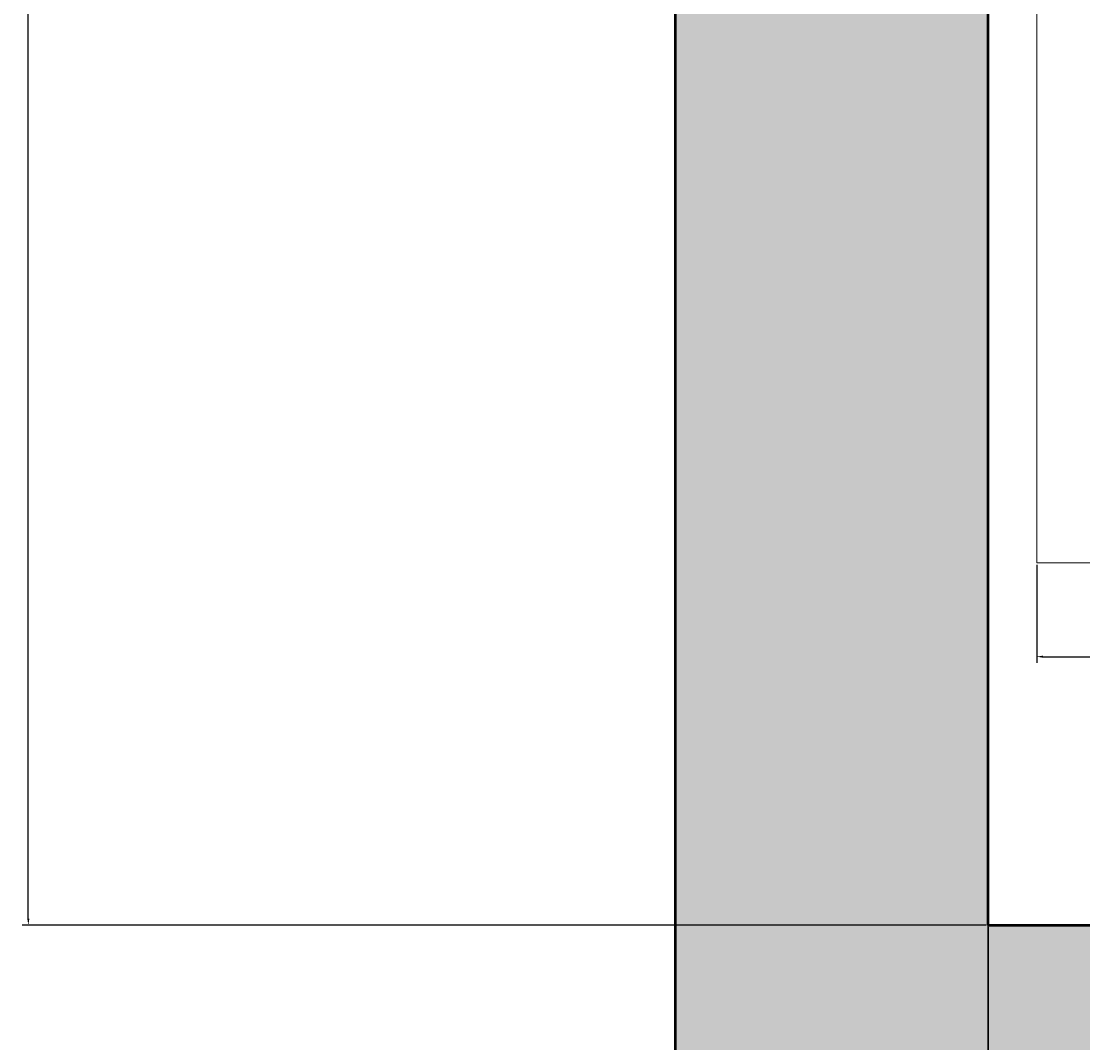
# Model space of a CAD drawing. Units: inches. Extents: x 2231 to 2461, y 2045 to 2455.
# Tile 50 of 95: x 2231 to 2262, y 2303 to 2333. Entities that reach past the tile are written whole.
import ezdxf

# ---------------------------------------------------------------- set-up
doc = ezdxf.new("R2010")
doc.units = ezdxf.units.IN
for name, color, linetype, lineweight in [('A-ANNO-DIMS', 2, 'Continuous', 18), ('A-FURN', 9, 'Continuous', 18), ('A-WALL', 7, 'Continuous', 50)]:
    doc.layers.add(name, color=color, linetype=linetype, lineweight=lineweight)
doc.layers.add('A-WALL-PATT', color=18, linetype='Continuous', lineweight=13, true_color=0x000000)
doc.styles.get("Standard").update_dxf_attribs({"font": 'arial.ttf'})
doc.dimstyles.get("Standard").update_dxf_attribs({"dimtxt": 0.18, "dimasz": 0.18, "dimexe": 0.18, "dimexo": 0.0625, "dimgap": 0.09, "dimtad": 0, "dimtih": 1, "dimtoh": 1, "dimdec": 4, "dimzin": 0, "dimdsep": 46, "dimtxsty": 'Standard', "dimcen": 0.09, "dimadec": 0, "dimazin": 0, "dimtfac": 1, "dimtdec": 4, "dimtofl": 0, "dimtmove": 0, "dimatfit": 3, "dimfxl": 1, "dimtolj": 1, "dimtzin": 0, "dimarcsym": 0})

# ---------------------------------------------------------------- blocks, each defined once
blk = doc.blocks.new('NIGHTSTAND-18IN')
blk.add_lwpolyline([(0, 0), (18, 0), (18, 18), (0, 18)], close=True)
blk = doc.blocks.new('*D17')
at = {"layer": 'A-ANNO-DIMS', "color": 0, "lineweight": -2, "transparency": 16777216}
for p, q in [((2260.188, 2317.191), (2260.188, 2314.373)), ((2278.188, 2317.191), (2278.188, 2314.373)), ((2260.368, 2314.553), (2267.812, 2314.553)), ((2278.008, 2314.553), (2270.564, 2314.553))]:
    blk.add_line(p, q, dxfattribs=at)
at = {"layer": 'A-ANNO-DIMS', "color": 0, "transparency": 16777216}
for points in [[(2260.368, 2314.583), (2260.368, 2314.523), (2260.188, 2314.553)], [(2278.008, 2314.583), (2278.008, 2314.523), (2278.188, 2314.553)]]:
    blk.add_solid(points, dxfattribs=at)
at = {"layer": 'Defpoints', "color": 0, "transparency": 16777216}
for p in [(2260.188, 2317.253), (2278.188, 2317.253), (2278.188, 2314.553)]:
    blk.add_point(p, dxfattribs=at)
at = {"layer": 'A-ANNO-DIMS', "color": 0, "transparency": 16777216, "insert": (2269.188, 2314.553), "char_height": 0.18, "attachment_point": 5}
blk.add_mtext('\\A1;NIGHTSTAND 18 TYP.', dxfattribs=at)
blk = doc.blocks.new('*D37')
at = {"layer": 'A-ANNO-DIMS', "color": 0, "lineweight": -2, "transparency": 16777216}
for p, q in [((2258.731, 2426.833), (2230.981, 2426.833)), ((2231.161, 2426.653), (2231.161, 2367.015)), ((2231.161, 2307.013), (2231.161, 2366.651)), ((2258.731, 2306.833), (2230.981, 2306.833))]:
    blk.add_line(p, q, dxfattribs=at)
at = {"layer": 'A-ANNO-DIMS', "color": 0, "transparency": 16777216}
for points in [[(2231.131, 2426.653), (2231.191, 2426.653), (2231.161, 2426.833)], [(2231.131, 2307.013), (2231.191, 2307.013), (2231.161, 2306.833)]]:
    blk.add_solid(points, dxfattribs=at)
at = {"layer": 'Defpoints', "color": 0, "transparency": 16777216}
for p in [(2231.161, 2426.833), (2258.794, 2426.833), (2258.794, 2306.833)]:
    blk.add_point(p, dxfattribs=at)
at = {"layer": 'A-ANNO-DIMS', "color": 0, "transparency": 16777216, "insert": (2231.161, 2366.833), "char_height": 0.18, "attachment_point": 5}
blk.add_mtext('\\A1;120', dxfattribs=at)
blk = doc.blocks.new('*D47')
at = {"layer": 'A-ANNO-DIMS', "color": 0, "lineweight": -2, "transparency": 16777216}
for p, q in [((2258.794, 2182.895), (2258.794, 2454.645)), ((2258.974, 2454.465), (2276.575, 2454.465)), ((2294.614, 2454.465), (2277.012, 2454.465)), ((2294.794, 2182.895), (2294.794, 2454.645))]:
    blk.add_line(p, q, dxfattribs=at)
at = {"layer": 'A-ANNO-DIMS', "color": 0, "transparency": 16777216}
for points in [[(2258.974, 2454.495), (2258.974, 2454.435), (2258.794, 2454.465)], [(2294.614, 2454.495), (2294.614, 2454.435), (2294.794, 2454.465)]]:
    blk.add_solid(points, dxfattribs=at)
at = {"layer": 'Defpoints', "color": 0, "transparency": 16777216}
for p in [(2294.794, 2454.465), (2258.794, 2182.833), (2294.794, 2182.833)]:
    blk.add_point(p, dxfattribs=at)
at = {"layer": 'A-ANNO-DIMS', "color": 0, "transparency": 16777216, "insert": (2276.794, 2454.465), "char_height": 0.18, "attachment_point": 5}
blk.add_mtext('\\A1;36', dxfattribs=at)
blk = doc.blocks.new('*D51')
at = {"layer": 'A-ANNO-DIMS', "color": 0, "lineweight": -2, "transparency": 16777216}
for p, q in [((2258.794, 2306.77), (2258.794, 2044.803)), ((2330.794, 2306.77), (2330.794, 2044.803)), ((2258.974, 2044.983), (2294.576, 2044.983)), ((2330.614, 2044.983), (2295.011, 2044.983))]:
    blk.add_line(p, q, dxfattribs=at)
at = {"layer": 'A-ANNO-DIMS', "color": 0, "transparency": 16777216}
for points in [[(2258.974, 2045.013), (2258.974, 2044.953), (2258.794, 2044.983)], [(2330.614, 2045.013), (2330.614, 2044.953), (2330.794, 2044.983)]]:
    blk.add_solid(points, dxfattribs=at)
at = {"layer": 'Defpoints', "color": 0, "transparency": 16777216}
for p in [(2258.794, 2306.833), (2330.794, 2306.833), (2330.794, 2044.983)]:
    blk.add_point(p, dxfattribs=at)
at = {"layer": 'A-ANNO-DIMS', "color": 0, "transparency": 16777216, "insert": (2294.794, 2044.983), "char_height": 0.18, "attachment_point": 5}
blk.add_mtext('\\A1;72', dxfattribs=at)

msp = doc.modelspace()

# ---------------------------------------------------------------- hatches: boundary and pattern name
at = {"layer": 'A-WALL-PATT'}
h = msp.add_hatch(color=256, dxfattribs=at)
h.dxf.hatch_style = 1
h.paths.add_polyline_path([(2441.7935, 2269.1535), (2432.7935, 2269.1535), (2432.7935, 2186.8328), (2396.7935, 2186.8328), (2396.7935, 2286.8328), (2394.7935, 2286.8328), (2394.7935, 2186.8328), (2334.7935, 2186.8328), (2334.7935, 2182.8328), (2432.7935, 2182.8328), (2432.7935, 2072.8328), (2416.6639, 2072.8328), (2416.6639, 2063.8328), (2441.7935, 2063.8328)])
h.paths.add_polyline_path([(2368.6639, 2072.8328), (2367.04, 2072.8328), (2330.7942, 2072.8328), (2330.7397, 2063.8328), (2368.6639, 2063.8328)])
h.paths.add_polyline_path([(2300.7392, 2068.3328), (2300.7392, 2072.8328), (2298.7935, 2072.8328), (2294.7935, 2072.8328), (2258.7935, 2072.8328), (2258.7935, 2120.8328), (2294.7935, 2120.8328), (2298.7935, 2120.8328), (2298.7935, 2128.8328), (2294.7935, 2128.8328), (2294.7935, 2124.8328), (2258.7935, 2124.8328), (2258.7935, 2182.8328), (2294.7935, 2182.8328), (2294.7935, 2174.8328), (2298.7935, 2174.8328), (2298.7935, 2182.8328), (2304.7935, 2182.8328), (2304.7935, 2186.8328), (2258.7935, 2186.8328), (2258.7935, 2221.999), (2249.7935, 2221.999), (2249.7935, 2063.8328), (2300.7392, 2063.8328)])
h.paths.add_polyline_path([(2391.9338, 2435.8328), (2333.82, 2435.8328), (2333.82, 2426.8328), (2368.7935, 2426.8328), (2368.7935, 2374.9508), (2368.7935, 2370.8328), (2372.3935, 2370.8328), (2372.7935, 2370.8328), (2372.7935, 2426.8328), (2391.9338, 2426.8328)])
h.paths.add_polyline_path([(2441.7935, 2435.8328), (2415.9338, 2435.8328), (2415.9338, 2426.8328), (2432.7935, 2426.8328), (2432.7935, 2334.8328), (2372.7935, 2334.8328), (2372.7935, 2346.8328), (2368.7935, 2346.8328), (2368.7935, 2306.8328), (2360.7935, 2306.8328), (2360.7935, 2302.8328), (2368.7935, 2302.8328), (2372.7935, 2302.8328), (2372.7935, 2330.8328), (2432.7935, 2330.8328), (2432.7935, 2317.1535), (2441.7935, 2317.1535)])
h.paths.add_polyline_path([(2285.82, 2435.8328), (2249.7935, 2435.8328), (2249.7935, 2269.999), (2258.7935, 2269.999), (2258.7935, 2302.8328), (2318.8168, 2302.8328), (2330.7935, 2302.8328), (2330.7935, 2306.8328), (2258.7935, 2306.8328), (2258.7935, 2426.8328), (2285.82, 2426.8328)])

# ---------------------------------------------------------------- linework, layer by layer
at = {"layer": 'A-WALL'}
for q in [(2258.7935, 2426.8328), (2330.7935, 2306.8328)]:
    msp.add_line((2258.7935, 2306.8328), q, dxfattribs=at)
msp.add_lwpolyline([(2300.7392, 2063.8328), (2249.7935, 2063.8328), (2249.7935, 2435.8328), (2441.7935, 2435.8328), (2441.7935, 2063.8328), (2330.7397, 2063.8328)], dxfattribs=at)

# ---------------------------------------------------------------- block references
at = {"layer": 'A-FURN'}
msp.add_blockref('NIGHTSTAND-18IN', (2260.188, 2317.253), dxfattribs=at)

# ---------------------------------------------------------------- dimensions: what is measured, and where the dimension line sits
at = {"layer": 'A-ANNO-DIMS'}
for base, p1, p2, picture, middle in [((2294.7935, 2454.4653), (2258.7935, 2182.8328), (2294.7935, 2182.8328), '*D47', (2276.7935, 2454.4653)), ((2330.7935, 2044.9825), (2258.7935, 2306.8328), (2330.7935, 2306.8328), '*D51', (2294.7935, 2044.9825))]:
    dim = msp.add_linear_dim(base=base, p1=p1, p2=p2, dimstyle='Standard', override={"dimdec": 0, "dimlfac": 1, "dimrnd": 0, "dimzin": 0, "dimdsep": 46, "dimlunit": 2}, dxfattribs=at)
    dim.commit()
    dim.dimension.update_dxf_attribs({"geometry": picture, "text_midpoint": middle})
dim = msp.add_linear_dim(base=(2231.161, 2426.8328), p1=(2258.7935, 2306.8328), p2=(2258.7935, 2426.8328), angle=90, dimstyle='Standard', override={"dimdec": 0, "dimlfac": 1, "dimrnd": 0, "dimzin": 0, "dimdsep": 46, "dimlunit": 2}, dxfattribs=at)
dim.commit()
dim.dimension.update_dxf_attribs({"geometry": '*D37', "text_midpoint": (2231.161, 2366.8328)})
dim = msp.add_linear_dim(base=(2278.1881, 2314.5534), p1=(2260.1881, 2317.2534), p2=(2278.1881, 2317.2534), text='NIGHTSTAND <> TYP.', dimstyle='Standard', override={"dimdec": 0, "dimlfac": 1, "dimrnd": 0, "dimzin": 0, "dimdsep": 46, "dimlunit": 2}, dxfattribs=at)
dim.commit()
dim.dimension.update_dxf_attribs({"geometry": '*D17', "text_midpoint": (2269.1881, 2314.5534)})

doc.saveas('drawing.dxf')
